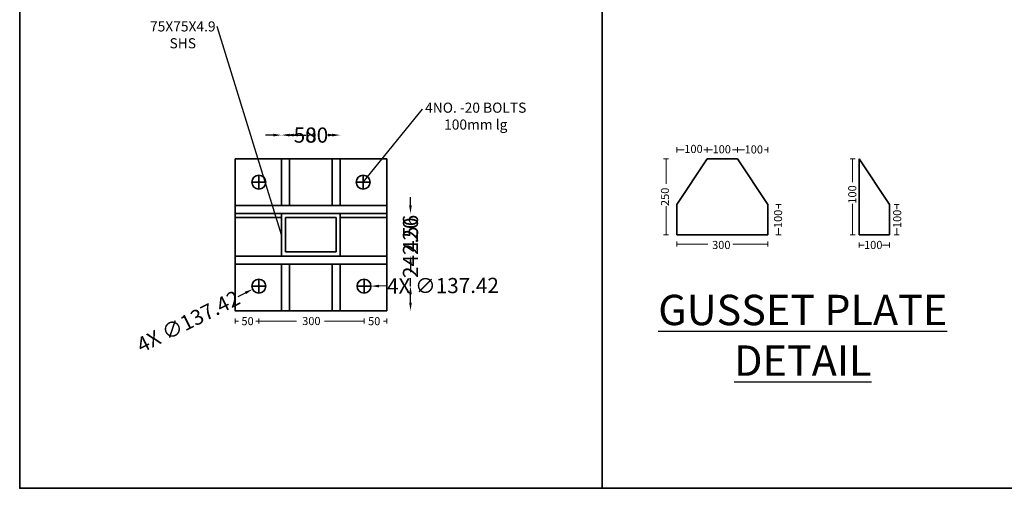
# Model space of a CAD drawing. Units: millimetres. Extents: x -19888 to 14444, y 67066 to 90098.
# Tile 1 of 7: x -19252 to -9513, y 69227 to 73856. Entities that reach past the tile are written whole.
import ezdxf
from ezdxf import colors
from ezdxf.entities.mleader import LeaderData, LeaderLine
from ezdxf.math import Vec2, Vec3

# ---------------------------------------------------------------- set-up
doc = ezdxf.new("R2010")
doc.units = ezdxf.units.MM
doc.header["$LTSCALE"] = 50
doc.header["$MEASUREMENT"] = 0
for name, color, linetype, lineweight in [('S-ANNO-DIMS', 2, 'Continuous', 18), ('S-ANNO-TEXT', 7, 'Continuous', 25), ('S-ANNO-TTLB', 7, 'Continuous', 35), ('S-STEL', 5, 'Continuous', 35)]:
    doc.layers.add(name, color=color, linetype=linetype, lineweight=lineweight)
doc.styles.get("Standard").update_dxf_attribs({"font": 'arial.ttf'})
doc.dimstyles.get("Standard").update_dxf_attribs({"dimtxt": 150, "dimasz": 80, "dimexe": 0.18, "dimexo": 0.0625, "dimgap": 0.09, "dimtad": 0, "dimdec": 0, "dimzin": 0, "dimdsep": 46, "dimtxsty": 'Standard', "dimcen": 0.09, "dimadec": 0, "dimazin": 0, "dimtfac": 1, "dimtdec": 0, "dimtofl": 0, "dimtmove": 0, "dimatfit": 3, "dimfxl": 1, "dimfxlon": 1, "dimtolj": 1, "dimtzin": 0, "dimarcsym": 0})

# ---------------------------------------------------------------- blocks, each defined once
blk = doc.blocks.new('BOLT-M20-PLAN')
at = {"ltscale": 50}
for p, q in [((68.7, 0), (68.7, 137.4)), ((137.4, 68.7), (0, 68.7))]:
    blk.add_line(p, q, dxfattribs=at)
blk.add_circle((68.7, 68.7), 68.7, dxfattribs=at)
blk = doc.blocks.new('*D46')
at = {"layer": 'Defpoints', "color": 0, "ltscale": 50, "transparency": 16777216}
for p in [(-15845.9, 71223.6), (-15386.3, 71223.6), (-15621.3, 70981.1)]:
    blk.add_point(p, dxfattribs=at)
at = {"layer": 'S-ANNO-DIMS', "color": 0, "lineweight": -2, "ltscale": 50, "transparency": 16777216}
for p, q in [((-15386.3, 71223.6), (-15386.3, 71303.6)), ((-15387.3, 71223.6), (-15386.1, 71223.6)), ((-15386.3, 71061.1), (-15386.3, 71143.6)), ((-15387.3, 70981.1), (-15386.1, 70981.1))]:
    blk.add_line(p, q, dxfattribs=at)
at = {"layer": 'S-ANNO-DIMS', "color": 0, "ltscale": 50, "transparency": 16777216}
for points in [[(-15399.6, 71143.6), (-15372.9, 71143.6), (-15386.3, 71223.6)], [(-15399.6, 71061.1), (-15372.9, 71061.1), (-15386.3, 70981.1)]]:
    blk.add_solid(points, dxfattribs=at)
at = {"layer": 'S-ANNO-DIMS', "color": 0, "ltscale": 50, "transparency": 16777216, "insert": (-15386.3, 71616.3), "char_height": 150, "attachment_point": 5, "rotation": 90}
blk.add_mtext('\\A1;242.56', dxfattribs=at)
blk = doc.blocks.new('*D47')
at = {"layer": 'Defpoints', "color": 0, "ltscale": 50, "transparency": 16777216}
for p in [(-16081.3, 72716.1), (-16661.3, 71941.1), (-16081.3, 71941.1)]:
    blk.add_point(p, dxfattribs=at)
at = {"layer": 'S-ANNO-DIMS', "color": 0, "lineweight": -2, "ltscale": 50, "transparency": 16777216}
for p, q in [((-16661.3, 72715.1), (-16661.3, 72716.2)), ((-16581.3, 72716.1), (-16536.8, 72716.1)), ((-16161.3, 72716.1), (-16205.7, 72716.1)), ((-16081.3, 72715.1), (-16081.3, 72716.2))]:
    blk.add_line(p, q, dxfattribs=at)
at = {"layer": 'S-ANNO-DIMS', "color": 0, "ltscale": 50, "transparency": 16777216}
for points in [[(-16581.3, 72729.4), (-16581.3, 72702.7), (-16661.3, 72716.1)], [(-16161.3, 72729.4), (-16161.3, 72702.7), (-16081.3, 72716.1)]]:
    blk.add_solid(points, dxfattribs=at)
at = {"layer": 'S-ANNO-DIMS', "color": 0, "ltscale": 50, "transparency": 16777216, "insert": (-16371.3, 72716.1), "char_height": 150, "attachment_point": 5}
blk.add_mtext('\\A1;580', dxfattribs=at)
blk = doc.blocks.new('*D48')
at = {"layer": 'Defpoints', "color": 0, "ltscale": 50, "transparency": 16777216}
for p in [(-16081.3, 71941.1), (-16081.3, 71521.1), (-15386.3, 71521.1)]:
    blk.add_point(p, dxfattribs=at)
at = {"layer": 'S-ANNO-DIMS', "color": 0, "lineweight": -2, "ltscale": 50, "transparency": 16777216}
for p, q in [((-15386.3, 72021.1), (-15386.3, 72101.1)), ((-15387.3, 71941.1), (-15386.1, 71941.1)), ((-15387.3, 71521.1), (-15386.1, 71521.1)), ((-15386.3, 71441.1), (-15386.3, 71361.1))]:
    blk.add_line(p, q, dxfattribs=at)
at = {"layer": 'S-ANNO-DIMS', "color": 0, "ltscale": 50, "transparency": 16777216}
for points in [[(-15399.6, 72021.1), (-15372.9, 72021.1), (-15386.3, 71941.1)], [(-15399.6, 71441.1), (-15372.9, 71441.1), (-15386.3, 71521.1)]]:
    blk.add_solid(points, dxfattribs=at)
at = {"layer": 'S-ANNO-DIMS', "color": 0, "ltscale": 50, "transparency": 16777216, "insert": (-15386.3, 71731.1), "char_height": 150, "attachment_point": 5, "rotation": 90}
blk.add_mtext('\\A1;420', dxfattribs=at)
blk = doc.blocks.new('*D49')
at = {"layer": 'Defpoints', "color": 0, "ltscale": 50, "transparency": 16777216}
for p in [(-16581.3, 72716.1), (-16661.3, 72481.1), (-16581.3, 72481.1)]:
    blk.add_point(p, dxfattribs=at)
at = {"layer": 'S-ANNO-DIMS', "color": 0, "lineweight": -2, "ltscale": 50, "transparency": 16777216}
for p, q in [((-16741.3, 72716.1), (-16821.3, 72716.1)), ((-16661.3, 72715.1), (-16661.3, 72716.2)), ((-16581.3, 72715.1), (-16581.3, 72716.2)), ((-16501.3, 72716.1), (-16421.3, 72716.1))]:
    blk.add_line(p, q, dxfattribs=at)
at = {"layer": 'S-ANNO-DIMS', "color": 0, "ltscale": 50, "transparency": 16777216}
for points in [[(-16741.3, 72729.4), (-16741.3, 72702.7), (-16661.3, 72716.1)], [(-16501.3, 72729.4), (-16501.3, 72702.7), (-16581.3, 72716.1)]]:
    blk.add_solid(points, dxfattribs=at)
at = {"layer": 'S-ANNO-DIMS', "color": 0, "ltscale": 50, "transparency": 16777216, "insert": (-16313.9, 72716.1), "char_height": 150, "attachment_point": 5}
blk.add_mtext('\\A1;80', dxfattribs=at)
blk = doc.blocks.new('*D50')
at = {"layer": 'Defpoints', "color": 0, "ltscale": 50, "transparency": 16777216}
for p in [(-16121.3, 72716.1), (-16621.3, 71901.1), (-16121.3, 71901.1)]:
    blk.add_point(p, dxfattribs=at)
at = {"layer": 'S-ANNO-DIMS', "color": 0, "lineweight": -2, "ltscale": 50, "transparency": 16777216}
for p, q in [((-16621.3, 72715.1), (-16621.3, 72716.2)), ((-16541.3, 72716.1), (-16536.8, 72716.1)), ((-16201.3, 72716.1), (-16205.7, 72716.1)), ((-16121.3, 72715.1), (-16121.3, 72716.2))]:
    blk.add_line(p, q, dxfattribs=at)
at = {"layer": 'S-ANNO-DIMS', "color": 0, "ltscale": 50, "transparency": 16777216}
for points in [[(-16541.3, 72729.4), (-16541.3, 72702.7), (-16621.3, 72716.1)], [(-16201.3, 72729.4), (-16201.3, 72702.7), (-16121.3, 72716.1)]]:
    blk.add_solid(points, dxfattribs=at)
at = {"layer": 'S-ANNO-DIMS', "color": 0, "ltscale": 50, "transparency": 16777216, "insert": (-16371.3, 72716.1), "char_height": 150, "attachment_point": 5}
blk.add_mtext('\\A1;500', dxfattribs=at)
blk = doc.blocks.new('*D68')
at = {"layer": 'Defpoints', "color": 0, "ltscale": 50, "transparency": 16777216}
for p in [(-15914.6, 71223.2), (-15777.2, 71224.1)]:
    blk.add_point(p, dxfattribs=at)
at = {"layer": 'S-ANNO-DIMS', "color": 0, "lineweight": -2, "ltscale": 50, "transparency": 16777216}
for p, q in [((-15846, 71223.6), (-15845.8, 71223.6)), ((-15845.9, 71223.5), (-15845.9, 71223.7)), ((-15617.2, 71225.1), (-15697.2, 71224.6))]:
    blk.add_line(p, q, dxfattribs=at)
at = {"layer": 'S-ANNO-DIMS', "color": 0, "ltscale": 50, "transparency": 16777216}
blk.add_solid([(-15697.3, 71237.9), (-15697.1, 71211.2), (-15777.2, 71224.1)], dxfattribs=at)
at = {"layer": 'S-ANNO-DIMS', "color": 0, "ltscale": 50, "transparency": 16777216, "insert": (-15064.7, 71228.5), "char_height": 150, "attachment_point": 5, "rotation": 0.36119}
blk.add_mtext('\\A1;4X ∅137.42', dxfattribs=at)
blk = doc.blocks.new('*D103')
at = {"layer": 'Defpoints', "color": 0, "ltscale": 50, "transparency": 16777216}
for p in [(-16947.1, 71192.9), (-16824.1, 71254.3)]:
    blk.add_point(p, dxfattribs=at)
at = {"layer": 'S-ANNO-DIMS', "color": 0, "lineweight": -2, "ltscale": 50, "transparency": 16777216}
for p, q in [((-16885.7, 71223.6), (-16885.5, 71223.6)), ((-16885.6, 71223.5), (-16885.6, 71223.7)), ((-17090.2, 71121.4), (-17018.6, 71157.2))]:
    blk.add_line(p, q, dxfattribs=at)
at = {"layer": 'S-ANNO-DIMS', "color": 0, "ltscale": 50, "transparency": 16777216}
blk.add_solid([(-17024.6, 71169.1), (-17012.7, 71145.3), (-16947.1, 71192.9)], dxfattribs=at)
at = {"layer": 'S-ANNO-DIMS', "color": 0, "ltscale": 50, "transparency": 16777216, "insert": (-17584.5, 70874.6), "char_height": 150, "attachment_point": 5, "rotation": 26.53699}
blk.add_mtext('\\A1;4X ∅137.42', dxfattribs=at)

msp = doc.modelspace()

# ---------------------------------------------------------------- linework, layer by layer
at = {"layer": 'S-ANNO-DIMS', "ltscale": 50}
for p, q in [((-12752.275, 72545.305), (-12752.275, 72595.305)), ((-12752.275, 72570.305), (-12677.866, 72570.305)), ((-12452.275, 72570.305), (-12485.571, 72570.305)), ((-12452.275, 72545.305), (-12452.275, 72595.305)), ((-12452.275, 72570.305), (-12398.736, 72570.305)), ((-12152.275, 72570.305), (-12201.737, 72570.305)), ((-12152.275, 72545.305), (-12152.275, 72595.305)), ((-12152.275, 72570.305), (-12081.605, 72570.305)), ((-11852.275, 72570.305), (-11884.973, 72570.305)), ((-11852.275, 72545.305), (-11852.275, 72595.305)), ((-12833.182, 72480.506), (-12883.182, 72480.506)), ((-12858.182, 72480.506), (-12858.182, 72235.218)), ((-10988.564, 72480.506), (-11038.564, 72480.506)), ((-11013.564, 72480.506), (-11013.564, 72251.307)), ((-12858.182, 71730.506), (-12858.182, 72015.011)), ((-11771.368, 72030.506), (-11721.368, 72030.506)), ((-11746.368, 72030.506), (-11746.368, 71989.624)), ((-11013.564, 71730.506), (-11013.564, 72038.307)), ((-10601.454, 72030.506), (-10551.454, 72030.506)), ((-10576.454, 72030.506), (-10576.454, 71984.865)), ((-11746.368, 71730.506), (-11746.368, 71797.388)), ((-10576.454, 71730.506), (-10576.454, 71797.253)), ((-12833.182, 71730.506), (-12883.182, 71730.506)), ((-11771.368, 71730.506), (-11721.368, 71730.506)), ((-10988.564, 71730.506), (-11038.564, 71730.506)), ((-10601.454, 71730.506), (-10551.454, 71730.506)), ((-12752.275, 71663.902), (-12752.275, 71613.902)), ((-12752.275, 71638.902), (-12446.004, 71638.902)), ((-11852.275, 71638.902), (-12199.15, 71638.902)), ((-11852.275, 71663.902), (-11852.275, 71613.902)), ((-10949.303, 71654.203), (-10949.303, 71604.203)), ((-10949.303, 71629.203), (-10899.611, 71629.203)), ((-10649.303, 71629.203), (-10716.196, 71629.203)), ((-10649.303, 71654.203), (-10649.303, 71604.203)), ((-17121.256, 70904.136), (-17121.256, 70854.136)), ((-16885.587, 70904.136), (-16885.587, 70854.136)), ((-15845.899, 70904.136), (-15845.899, 70854.136)), ((-15621.256, 70904.136), (-15621.256, 70854.136)), ((-17121.256, 70879.136), (-17088.13, 70879.136)), ((-16885.587, 70879.136), (-16916.235, 70879.136)), ((-16885.587, 70879.136), (-16515.116, 70879.136)), ((-15845.899, 70879.136), (-16238.288, 70879.136)), ((-15621.256, 70879.136), (-15654.382, 70879.136))]:
    msp.add_line(p, q, dxfattribs=at)
at = {"layer": 'S-ANNO-TTLB', "ltscale": 50}
for points in [[(-19251.506, 74235.431), (-13491.006, 74235.431), (-13491.006, 69226.696), (-19251.506, 69226.696)], [(-13491.006, 74235.431), (-9009.653, 74235.431), (-9009.653, 69226.696), (-13491.006, 69226.696)]]:
    msp.add_lwpolyline(points, close=True, dxfattribs=at)
at = {"layer": 'S-STEL', "ltscale": 50}
for p, q in [((-16661.256, 72481.064), (-16661.256, 72021.064)), ((-16581.256, 72481.064), (-16581.256, 72021.064)), ((-16161.256, 72481.064), (-16161.256, 72021.064)), ((-16081.256, 72481.064), (-16081.256, 72021.064)), ((-15621.256, 72481.064), (-15621.256, 70981.064)), ((-12452.275, 72480.506), (-12752.275, 72030.506)), ((-12452.275, 72480.506), (-12152.275, 72480.506)), ((-11852.275, 72030.506), (-12152.275, 72480.506)), ((-10949.303, 71730.506), (-10949.303, 72480.506)), ((-10949.303, 72480.506), (-10649.303, 72030.506)), ((-15621.256, 72021.064), (-17121.256, 72021.064)), ((-12752.275, 71730.506), (-12752.275, 72030.506)), ((-11852.275, 71730.506), (-11852.275, 72030.506)), ((-10649.303, 71730.506), (-10649.303, 72030.506)), ((-15621.256, 71941.064), (-17121.256, 71941.064)), ((-16661.256, 71901.064), (-17121.256, 71901.064)), ((-16661.256, 71941.064), (-16661.256, 71521.064)), ((-16621.256, 71901.064), (-16621.256, 71561.064)), ((-16121.256, 71901.064), (-16621.256, 71901.064)), ((-16121.256, 71901.064), (-16121.256, 71561.064)), ((-16081.256, 71941.064), (-16081.256, 71521.064)), ((-15621.256, 71901.064), (-16081.256, 71901.064)), ((-12752.275, 71730.506), (-11852.275, 71730.506)), ((-10949.303, 71730.506), (-10649.303, 71730.506)), ((-16661.256, 71521.064), (-17121.256, 71521.064)), ((-16081.256, 71521.064), (-16661.256, 71521.064)), ((-16121.256, 71561.064), (-16621.256, 71561.064)), ((-15621.256, 71521.064), (-16081.256, 71521.064)), ((-15621.256, 71441.064), (-17121.256, 71441.064)), ((-16661.256, 71441.064), (-16661.256, 70981.064)), ((-16581.256, 71441.064), (-16581.256, 70981.064)), ((-16161.256, 71441.064), (-16161.256, 70981.064)), ((-16081.256, 71441.064), (-16081.256, 70981.064))]:
    msp.add_line(p, q, dxfattribs=at)
msp.add_lwpolyline([(-17121.256, 72481.064), (-15621.256, 72481.064), (-15621.256, 70981.064), (-17121.256, 70981.064)], close=True, dxfattribs=at)

# ---------------------------------------------------------------- block references
at = {"layer": 'S-STEL'}
for p in [(-16954.296, 72182.354), (-15923.131, 72182.354), (-16954.296, 71154.913), (-15914.608, 71154.913)]:
    msp.add_blockref('BOLT-M20-PLAN', p, dxfattribs=at)

# ---------------------------------------------------------------- texts
at = {"layer": 'S-ANNO-TEXT', "ltscale": 50}
for s, width, gutter_width, insert, char_height, attachment_point in [('100', 839.57537, 0.522, (-12677.866, 72619.058), 80, 1), ('100', 839.57537, 0.522, (-12398.736, 72615.926), 80, 1), ('100', 839.57537, 0.522, (-12081.605, 72614.029), 80, 1), ('300', 839.57537, 0.522, (-12402.931, 71670.547), 80, 1), ('100', 839.57537, 0.522, (-10899.959, 71670.547), 80, 1), ('\\pxqc;{\\LGUSSET PLATE\\PDETAIL}', 3602.83103, 1, (-13307.715, 71138.212), 300, 1), ('50', 839.57537, 0.522, (-17058.143, 70917.642), 80, 1), ('300', 839.57537, 0.522, (-16457.558, 70919.062), 80, 1), ('50', 839.57537, 0.522, (-15684.368, 70917.642), 80, 3)]:
    msp.add_mtext_dynamic_manual_height_columns(s, width=width, gutter_width=gutter_width, heights=[0], dxfattribs=dict(at, insert=insert, char_height=char_height, attachment_point=attachment_point))
at = {"layer": 'S-ANNO-TEXT', "ltscale": 50, "char_height": 80, "attachment_point": 1, "rotation": 90}
for s, insert in [('250', (-12909.142, 72015.011)), ('100', (-11056.635, 72038.307)), ('100', (-11790.686, 71797.388)), ('100', (-10612.418, 71797.253))]:
    msp.add_mtext_dynamic_manual_height_columns(s, width=839.57537, gutter_width=0.522, heights=[0], dxfattribs=dict(at, insert=insert))

# ---------------------------------------------------------------- dimensions: what is measured, and where the dimension line sits
at = {"layer": 'S-ANNO-DIMS', "ltscale": 50}
for base, p1, p2, picture, middle in [((-16581.256, 72716.064), (-16661.256, 72481.064), (-16581.256, 72481.064), '*D49', (-16313.884, 72716.064)), ((-16081.256, 72716.064), (-16661.256, 71941.064), (-16081.256, 71941.064), '*D47', (-16371.256, 72716.064)), ((-16121.256, 72716.064), (-16621.256, 71901.064), (-16121.256, 71901.064), '*D50', (-16371.256, 72716.064))]:
    dim = msp.add_linear_dim(base=base, p1=p1, p2=p2, dimstyle='Standard', override={"dimdec": 0, "dimlfac": 1, "dimrnd": 0, "dimzin": 0, "dimdsep": 46, "dimlunit": 2}, dxfattribs=at)
    dim.commit()
    dim.dimension.update_dxf_attribs({"geometry": picture, "text_midpoint": middle})
for base, p1, p2, override, picture, middle in [((-15386.256, 71521.064), (-16081.256, 71941.064), (-16081.256, 71521.064), {"dimdec": 0, "dimlfac": 1, "dimrnd": 0, "dimzin": 0, "dimdsep": 46, "dimlunit": 2}, '*D48', (-15386.256, 71731.064)), ((-15386.256, 71223.622), (-15621.256, 70981.064), (-15845.899, 71223.622), {"dimdec": 2, "dimlfac": 1, "dimrnd": 0, "dimzin": 0, "dimdsep": 46, "dimlunit": 2}, '*D46', (-15386.256, 71616.298))]:
    dim = msp.add_linear_dim(base=base, p1=p1, p2=p2, angle=90, dimstyle='Standard', override=override, dxfattribs=at)
    dim.commit()
    dim.dimension.update_dxf_attribs({"geometry": picture, "text_midpoint": middle})
dim = msp.add_diameter_dim_2p(p1=(-15914.607, 71223.189), p2=(-15777.191, 71224.056), text='4X <>', dimstyle='Standard', override={"dimdec": 2, "dimlfac": 1, "dimrnd": 0, "dimzin": 0, "dimdsep": 46, "dimlunit": 2}, dxfattribs=at)
dim.commit()
dim.dimension.update_dxf_attribs({"geometry": '*D68', "text_midpoint": (-15064.745, 71228.547), "dimtype": 163})
dim = msp.add_diameter_dim_2p(p1=(-16824.117, 71254.32), p2=(-16947.057, 71192.925), text='4X <>', dimstyle='Standard', override={"dimdec": 2, "dimlfac": 1, "dimrnd": 0, "dimzin": 0, "dimdsep": 46, "dimlunit": 2}, dxfattribs=at)
dim.commit()
dim.dimension.update_dxf_attribs({"geometry": '*D103', "text_midpoint": (-17584.457, 70874.615)})

# ---------------------------------------------------------------- leaders
at = {"layer": 'S-ANNO-TEXT', "ltscale": 50}
ml = msp.add_multileader_mtext('Standard', dxfattribs=at)
ml.set_content('75X75X4.9\\PSHS', color=256)
ml.set_leader_properties()
ml.build(insert=Vec2(0, 0))
ml.multileader.update_dxf_attribs({"dogleg_length": 0.36, "arrow_head_size": 0.18})
ctx = ml.context
ctx.base_point, ctx.char_height, ctx.arrow_head_size, ctx.landing_gap_size, ctx.plane_origin = Vec3(-17977.669, 73788.735), 100, 0.18, 0.09, Vec3(-16661.256, 71731.064)
ctx.text_align_type = 1
notes = []
notes.append((ctx, [(0, (1, 1, 0), (-17298.548, 73788.735), (-1, 0), 0.36, [(0, [(-16661.256, 71731.064)], 0, [])])]))
ctx.mtext.insert, ctx.mtext.alignment, ctx.mtext.flow_direction = Vec3(-17638.288, 73839.588), 2, 5
ml = msp.add_multileader_mtext('Standard', dxfattribs=at)
ml.set_content('4NO. -20 BOLTS\\P100mm lg', color=256)
ml.set_leader_properties()
ml.build(insert=Vec2(0, 0))
ml.multileader.update_dxf_attribs({"dogleg_length": 0.36, "arrow_head_size": 0.18})
ctx = ml.context
ctx.base_point, ctx.char_height, ctx.arrow_head_size, ctx.landing_gap_size, ctx.plane_origin = Vec3(-15268.151, 72972.022), 100, 0.18, 0.09, Vec3(-15854.422, 72251.064)
ctx.text_align_type = 1
notes.append((ctx, [(0, (1, 1, 0), (-15268.511, 72972.022), (1, 0), 0.36, [(0, [(-15854.422, 72251.064)], 0, [])])]))
ctx.mtext.insert, ctx.mtext.alignment, ctx.mtext.flow_direction = Vec3(-14740.775, 73036.722), 2, 5
for ctx, leaders in notes:
    for number, flags, end, landing, length, lines in leaders:
        leader = LeaderData()
        leader.index, (leader.has_last_leader_line, leader.has_dogleg_vector, leader.attachment_direction) = number, flags
        leader.last_leader_point, leader.dogleg_vector, leader.dogleg_length = Vec3(end), Vec3(landing), length
        for number, points, colour, breaks in lines:
            line = LeaderLine()
            line.index, line.vertices, line.color, line.breaks = number, Vec3.list(points), colors.encode_raw_color(colour), breaks
            leader.lines.append(line)
        ctx.leaders.append(leader)

doc.saveas('drawing.dxf')
